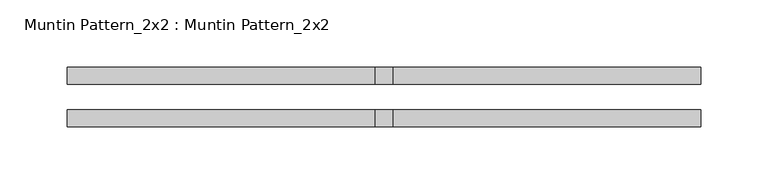
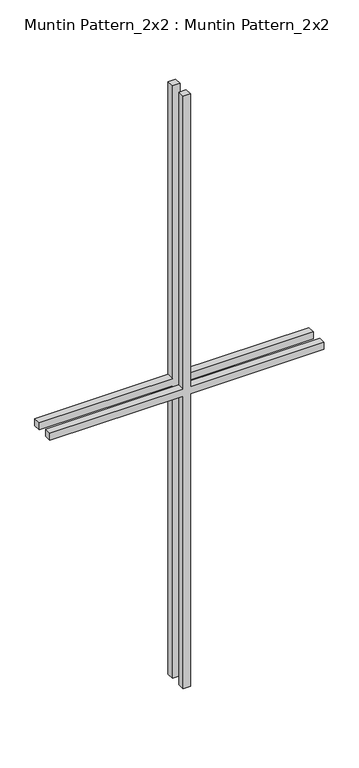
"""IFC4 building model written with IfcOpenShell, lengths in millimetres: proxy geometry, Muntin Pattern_2x2 : Muntin Pattern_2x2."""

from ifc_helpers import new_model, si_unit, frame, origin, place, context, project, spatial, polyline, outline, extrude, source, transform, mapped, element, save


def muntin_pattern_2x2_muntin_pattern_2x2_4dfeb3f3(model_context):
    return source(origin(), model_context, "Body", "SweptSolid", [
        extrude(outline(polyline([(546.1, -6.35), (546.1, -236.5375), (533.4, -236.5375), (533.4, -6.35), (0.0, -6.35), (0.0, 6.35), (533.4, 6.35), (533.4, 236.5375), (546.1, 236.5375), (546.1, 6.35), (1079.5, 6.35), (1079.5, -6.35), (546.1, -6.35)])), frame((0.0, 9.525, 0.0), z_axis=(0.0, 1.0, 0.0), x_axis=(0.0, 0.0, 1.0)), (0.0, 0.0, 1.0), 12.7),
        extrude(outline(polyline([(546.1, -6.35), (546.1, -236.5375), (533.4, -236.5375), (533.4, -6.35), (0.0, -6.35), (0.0, 6.35), (533.4, 6.35), (533.4, 236.5375), (546.1, 236.5375), (546.1, 6.35), (1079.5, 6.35), (1079.5, -6.35), (546.1, -6.35)])), frame((0.0, -22.225, 0.0), z_axis=(0.0, 1.0, 0.0), x_axis=(0.0, 0.0, 1.0)), (0.0, 0.0, 1.0), 12.7),
    ])


if __name__ == "__main__":
    model = new_model("IFC4")
    model_context = context("Model", 3, world=origin())
    ifc_project = project(units=[si_unit("LENGTHUNIT", "METRE", prefix="MILLI")], contexts=[model_context])
    site = spatial("IfcSite", under=ifc_project)
    building = spatial("IfcBuilding", under=site)
    placement = place(None, origin())
    muntin_pattern_2x2_muntin_pattern_2x2_shape = muntin_pattern_2x2_muntin_pattern_2x2_4dfeb3f3(model_context)
    element("IfcBuildingElementProxy", 1, Name="Muntin Pattern_2x2 : Muntin Pattern_2x2", ObjectType="Muntin Pattern_2x2 : Muntin Pattern_2x2", at=placement, inside=building, context=model_context, shape_type="MappedRepresentation", body=[
        mapped(muntin_pattern_2x2_muntin_pattern_2x2_shape, transform((0.0, 0.0, 0.0), x_axis=(1.0, 0.0, 0.0), y_axis=(0.0, 1.0, 0.0), z_axis=(0.0, 0.0, 1.0))),
    ])
    save(model, "model.ifc")

# Revit data of these elements
# Type "Muntin Pattern_2x2 : Muntin Pattern_2x2"
#   Width [instance default] = 4' - 0"
#   Thickness = 0' - 0 1/2"
#   Height [instance default] = 4' - 0"
#   Distance = 0' - 0 3/4"
#   Interior Material [instance default] = none
#   Exterior Material [instance default] = none
#   Default Elevation = 0
# Element 1 (IfcBuildingElementProxy, "Muntin Pattern_2x2 : Muntin Pattern_2x2")
#   Width = 1' - 6 5/8"
#   Height = 3' - 6 1/2"
#   Interior Material = Wood - Stained
#   Exterior Material = Clad - White
#   Materials on its faces: "Clad - White", "Wood - Stained"
# Materials
#   "Clad - White": class "Wood", colour RGB 242 242 238, transparency 0, Cost = 0
#   "Wood - Stained": class "Wood", colour RGB 224 178 126, transparency 0, Cost = 0
